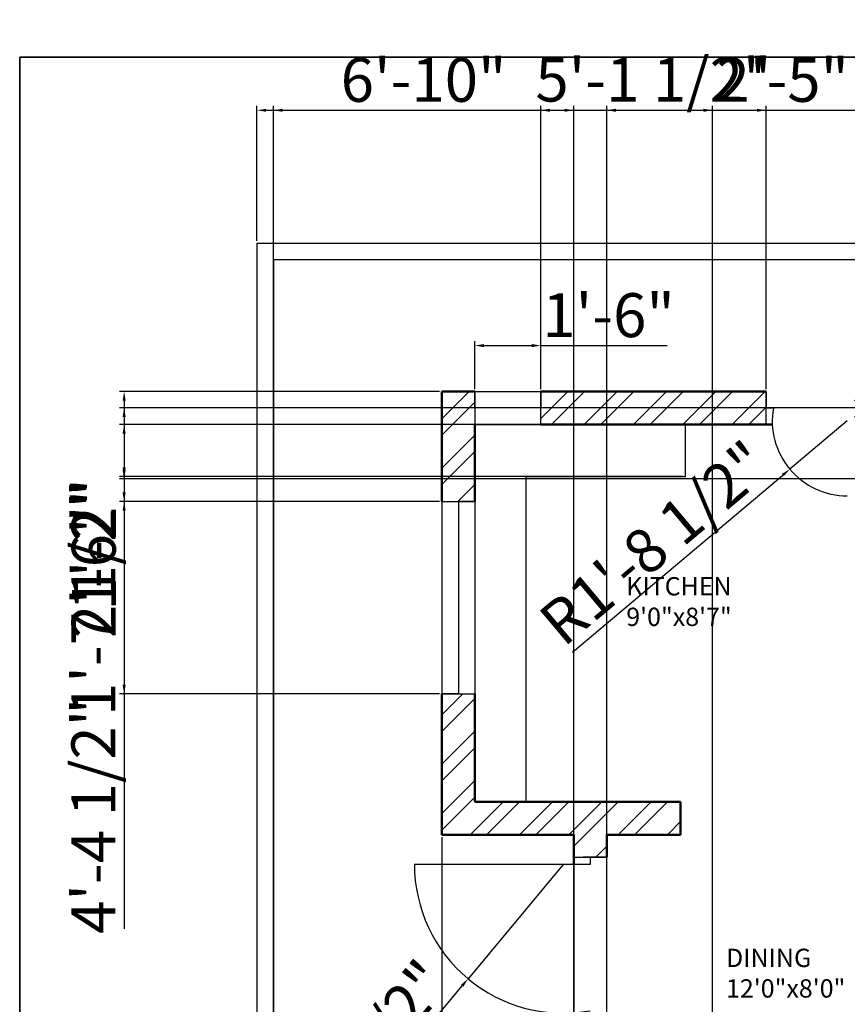
# Model space of a CAD drawing. Units: inches. Extents: x 1990 to 2869, y 1755 to 2533.
# Tile 2 of 6: x 1990 to 2216, y 2120 to 2389. Entities that reach past the tile are written whole.
import ezdxf

# ---------------------------------------------------------------- set-up
doc = ezdxf.new("R2010")
doc.units = ezdxf.units.IN
for name, color, linetype, lineweight in [('A-ANNO-DIMS', 171, 'Continuous', 18), ('A-ANNO-TTLB', 7, 'Continuous', 35), ('A-AREA-IDEN', 7, 'Continuous', 18), ('A-DOOR', 11, 'Continuous', 25), ('A-FLOR-CASE', 7, 'Continuous', 25), ('A-GLAZ', 121, 'Continuous', 25), ('A-WALL', 7, 'Continuous', 50), ('A-WALL-SITE', 7, 'Continuous', 30)]:
    doc.layers.add(name, color=color, linetype=linetype, lineweight=lineweight)
doc.layers.add('A-WALL-PATT', color=215, linetype='Continuous', lineweight=13, true_color=0xa953a0)
doc.styles.get("Standard").update_dxf_attribs({"font": 'arial.ttf'})
doc.dimstyles.new('ISO-25', dxfattribs={"dimtxt": 12, "dimasz": 2.5, "dimexe": 1.25, "dimexo": 0.625, "dimtad": 1, "dimdec": 0, "dimlunit": 3, "dimtxsty": 'Standard', "dimcen": 2.5, "dimadec": 0, "dimazin": 0, "dimtfac": 1, "dimtdec": 0, "dimtmove": 0, "dimatfit": 3, "dimfxl": 1, "dimarcsym": 0})

# ---------------------------------------------------------------- blocks, each defined once
blk = doc.blocks.new('*D2')
at = {"layer": 'A-ANNO-DIMS', "color": 0, "lineweight": -2, "transparency": 16777216}
for p, q in [((2113.97, 2288.18), (2113.97, 2301.32)), ((2131.97, 2288.18), (2131.97, 2301.32)), ((2116.47, 2300.07), (2129.47, 2300.07)), ((2131.97, 2300.07), (2166.49, 2300.07))]:
    blk.add_line(p, q, dxfattribs=at)
at = {"layer": 'A-ANNO-DIMS', "color": 0, "transparency": 16777216}
for points in [[(2116.47, 2300.49), (2116.47, 2299.65), (2113.97, 2300.07)], [(2129.47, 2300.49), (2129.47, 2299.65), (2131.97, 2300.07)]]:
    blk.add_solid(points, dxfattribs=at)
at = {"layer": 'Defpoints', "color": 0, "transparency": 16777216}
for p in [(2131.97, 2300.07), (2113.97, 2287.55), (2131.97, 2287.55)]:
    blk.add_point(p, dxfattribs=at)
at = {"layer": 'A-ANNO-DIMS', "color": 0, "transparency": 16777216, "insert": (2150.48, 2306.82), "char_height": 12, "attachment_point": 5}
blk.add_mtext('1\'-6"', dxfattribs=at)
blk = doc.blocks.new('WIN-18IN')
for p, q in [((0, 4.5), (0, 9)), ((0, 9), (0, 0)), ((0, 9), (18, 9)), ((18, 0), (18, 9)), ((18, 9), (18, 4.5)), ((18, 4.5), (0, 4.5)), ((0, 0), (18, 0))]:
    blk.add_line(p, q)
blk = doc.blocks.new('*D24')
at = {"layer": 'A-ANNO-DIMS', "color": 0, "lineweight": -2, "transparency": 16777216}
for p, q in [((2149.97, 1894.18), (2149.97, 2365.55)), ((2178.84, 1894.18), (2178.84, 2365.55)), ((2152.47, 2364.3), (2176.34, 2364.3)), ((2178.84, 2364.3), (2214.69, 2364.3))]:
    blk.add_line(p, q, dxfattribs=at)
at = {"layer": 'A-ANNO-DIMS', "color": 0, "transparency": 16777216}
for points in [[(2152.47, 2364.72), (2152.47, 2363.88), (2149.97, 2364.3)], [(2176.34, 2364.72), (2176.34, 2363.88), (2178.84, 2364.3)]]:
    blk.add_solid(points, dxfattribs=at)
at = {"layer": 'Defpoints', "color": 0, "transparency": 16777216}
for p in [(2178.84, 2364.3), (2149.97, 1893.55), (2178.84, 1893.55)]:
    blk.add_point(p, dxfattribs=at)
at = {"layer": 'A-ANNO-DIMS', "color": 0, "transparency": 16777216, "insert": (2198.02, 2371.05), "char_height": 12, "attachment_point": 5}
blk.add_mtext('2\'-5"', dxfattribs=at)
blk = doc.blocks.new('*D25')
at = {"layer": 'A-ANNO-DIMS', "color": 0, "lineweight": -2, "transparency": 16777216}
for p, q in [((2058.97, 1885.18), (2058.97, 2365.55)), ((2140.97, 1885.18), (2140.97, 2365.55)), ((2061.47, 2364.3), (2138.47, 2364.3))]:
    blk.add_line(p, q, dxfattribs=at)
at = {"layer": 'A-ANNO-DIMS', "color": 0, "transparency": 16777216}
for points in [[(2061.47, 2364.72), (2061.47, 2363.88), (2058.97, 2364.3)], [(2138.47, 2364.72), (2138.47, 2363.88), (2140.97, 2364.3)]]:
    blk.add_solid(points, dxfattribs=at)
at = {"layer": 'Defpoints', "color": 0, "transparency": 16777216}
for p in [(2140.97, 2364.3), (2058.97, 1884.55), (2140.97, 1884.55)]:
    blk.add_point(p, dxfattribs=at)
at = {"layer": 'A-ANNO-DIMS', "color": 0, "transparency": 16777216, "insert": (2099.97, 2371.05), "char_height": 12, "attachment_point": 5}
blk.add_mtext('6\'-10"', dxfattribs=at)
blk = doc.blocks.new('*D33')
at = {"layer": 'A-ANNO-DIMS', "color": 0, "lineweight": -2, "transparency": 16777216}
for p, q in [((2104.97, 2165.93), (2104.97, 1764.83)), ((2140.97, 2165.93), (2140.97, 1764.83)), ((2107.47, 1766.08), (2138.47, 1766.08))]:
    blk.add_line(p, q, dxfattribs=at)
at = {"layer": 'A-ANNO-DIMS', "color": 0, "transparency": 16777216}
for points in [[(2107.47, 1766.49), (2107.47, 1765.66), (2104.97, 1766.08)], [(2138.47, 1766.49), (2138.47, 1765.66), (2140.97, 1766.08)]]:
    blk.add_solid(points, dxfattribs=at)
at = {"layer": 'Defpoints', "color": 0, "transparency": 16777216}
for p in [(2104.97, 2166.55), (2140.97, 2166.55), (2140.97, 1766.08)]:
    blk.add_point(p, dxfattribs=at)
at = {"layer": 'A-ANNO-DIMS', "color": 0, "transparency": 16777216, "insert": (2122.97, 1772.83), "char_height": 12, "attachment_point": 5}
blk.add_mtext('3\'-0"', dxfattribs=at)
blk = doc.blocks.new('*D34')
at = {"layer": 'A-ANNO-DIMS', "color": 0, "lineweight": -2, "transparency": 16777216}
for p, q in [((2104.35, 2257.5), (2016.97, 2257.5)), ((2018.22, 2255), (2018.22, 2207.5)), ((2104.35, 2205), (2016.97, 2205)), ((2018.22, 2205), (2018.22, 2140.9))]:
    blk.add_line(p, q, dxfattribs=at)
at = {"layer": 'A-ANNO-DIMS', "color": 0, "transparency": 16777216}
for points in [[(2017.8, 2255), (2018.64, 2255), (2018.22, 2257.5)], [(2017.8, 2207.5), (2018.64, 2207.5), (2018.22, 2205)]]:
    blk.add_solid(points, dxfattribs=at)
at = {"layer": 'Defpoints', "color": 0, "transparency": 16777216}
for p in [(2104.97, 2257.5), (2018.22, 2205), (2104.97, 2205)]:
    blk.add_point(p, dxfattribs=at)
at = {"layer": 'A-ANNO-DIMS', "color": 0, "transparency": 16777216, "insert": (2011.39, 2171.7), "char_height": 12, "attachment_point": 5, "rotation": 90}
blk.add_mtext('4\'-4 1/2"', dxfattribs=at)
blk = doc.blocks.new('*D35')
at = {"layer": 'A-ANNO-DIMS', "color": 0, "lineweight": -2, "transparency": 16777216}
for p, q in [((2104.35, 2287.55), (2016.97, 2287.55)), ((2018.22, 2285.05), (2018.22, 2260)), ((2104.35, 2257.5), (2016.97, 2257.5)), ((2018.22, 2257.5), (2018.22, 2221.64))]:
    blk.add_line(p, q, dxfattribs=at)
at = {"layer": 'A-ANNO-DIMS', "color": 0, "transparency": 16777216}
for points in [[(2017.8, 2285.05), (2018.64, 2285.05), (2018.22, 2287.55)], [(2017.8, 2260), (2018.64, 2260), (2018.22, 2257.5)]]:
    blk.add_solid(points, dxfattribs=at)
at = {"layer": 'Defpoints', "color": 0, "transparency": 16777216}
for p in [(2104.97, 2287.55), (2018.22, 2257.5), (2104.97, 2257.5)]:
    blk.add_point(p, dxfattribs=at)
at = {"layer": 'A-ANNO-DIMS', "color": 0, "transparency": 16777216, "insert": (2011.47, 2238.32), "char_height": 12, "attachment_point": 5, "rotation": 90}
blk.add_mtext('2\'-6"', dxfattribs=at)
blk = doc.blocks.new('*D36')
at = {"layer": 'A-ANNO-DIMS', "color": 0, "lineweight": -2, "transparency": 16777216}
for p, q in [((2716.35, 2283.05), (2016.97, 2283.05)), ((2018.22, 2280.55), (2018.22, 2266.18)), ((2716.35, 2263.68), (2016.97, 2263.68)), ((2018.22, 2263.68), (2018.22, 2201.19))]:
    blk.add_line(p, q, dxfattribs=at)
at = {"layer": 'A-ANNO-DIMS', "color": 0, "transparency": 16777216}
for points in [[(2017.8, 2280.55), (2018.64, 2280.55), (2018.22, 2283.05)], [(2017.8, 2266.18), (2018.64, 2266.18), (2018.22, 2263.68)]]:
    blk.add_solid(points, dxfattribs=at)
at = {"layer": 'Defpoints', "color": 0, "transparency": 16777216}
for p in [(2716.97, 2283.05), (2018.22, 2263.68), (2716.97, 2263.68)]:
    blk.add_point(p, dxfattribs=at)
at = {"layer": 'A-ANNO-DIMS', "color": 0, "transparency": 16777216, "insert": (2011.39, 2231.19), "char_height": 12, "attachment_point": 5, "rotation": 90}
blk.add_mtext('1\'-7 1/2"', dxfattribs=at)
blk = doc.blocks.new('*D42')
at = {"layer": 'A-ANNO-DIMS', "color": 0, "lineweight": -2, "transparency": 16777216}
for p, q in [((2170.81, 2278.55), (2016.97, 2278.55)), ((2018.22, 2276.05), (2018.22, 2266.83)), ((2170.81, 2264.33), (2016.97, 2264.33)), ((2018.22, 2264.33), (2018.22, 2229.81))]:
    blk.add_line(p, q, dxfattribs=at)
at = {"layer": 'A-ANNO-DIMS', "color": 0, "transparency": 16777216}
for points in [[(2017.8, 2276.05), (2018.64, 2276.05), (2018.22, 2278.55)], [(2017.8, 2266.83), (2018.64, 2266.83), (2018.22, 2264.33)]]:
    blk.add_solid(points, dxfattribs=at)
at = {"layer": 'Defpoints', "color": 0, "transparency": 16777216}
for p in [(2171.44, 2278.55), (2018.22, 2264.33), (2171.44, 2264.33)]:
    blk.add_point(p, dxfattribs=at)
at = {"layer": 'A-ANNO-DIMS', "color": 0, "transparency": 16777216, "insert": (2011.57, 2245.82), "char_height": 12, "attachment_point": 5, "rotation": 90}
blk.add_mtext('1\'-2"', dxfattribs=at)
blk = doc.blocks.new('*D45')
at = {"layer": 'A-ANNO-DIMS', "color": 0, "lineweight": -2, "transparency": 16777216}
for p, q in [((2131.97, 2288.18), (2131.97, 2365.55)), ((2193.46, 2288.18), (2193.46, 2365.55)), ((2134.47, 2364.3), (2190.96, 2364.3))]:
    blk.add_line(p, q, dxfattribs=at)
at = {"layer": 'A-ANNO-DIMS', "color": 0, "transparency": 16777216}
for points in [[(2134.47, 2364.72), (2134.47, 2363.88), (2131.97, 2364.3)], [(2190.96, 2364.72), (2190.96, 2363.88), (2193.46, 2364.3)]]:
    blk.add_solid(points, dxfattribs=at)
at = {"layer": 'Defpoints', "color": 0, "transparency": 16777216}
for p in [(2193.46, 2364.3), (2131.97, 2287.55), (2193.46, 2287.55)]:
    blk.add_point(p, dxfattribs=at)
at = {"layer": 'A-ANNO-DIMS', "color": 0, "transparency": 16777216, "insert": (2162.72, 2371.13), "char_height": 12, "attachment_point": 5}
blk.add_mtext('5\'-1 1/2"', dxfattribs=at)
blk = doc.blocks.new('*D48')
at = {"layer": 'A-ANNO-DIMS', "color": 0, "lineweight": -2, "transparency": 16777216}
for p, q in [((2054.47, 2328.68), (2054.47, 2365.55)), ((2776.47, 2328.68), (2776.47, 2365.55)), ((2056.97, 2364.3), (2773.97, 2364.3))]:
    blk.add_line(p, q, dxfattribs=at)
at = {"layer": 'A-ANNO-DIMS', "color": 0, "transparency": 16777216}
for points in [[(2056.97, 2364.72), (2056.97, 2363.88), (2054.47, 2364.3)], [(2773.97, 2364.72), (2773.97, 2363.88), (2776.47, 2364.3)]]:
    blk.add_solid(points, dxfattribs=at)
at = {"layer": 'Defpoints', "color": 0, "transparency": 16777216}
for p in [(2776.47, 2364.3), (2054.47, 2328.05), (2776.47, 2328.05)]:
    blk.add_point(p, dxfattribs=at)
at = {"layer": 'A-ANNO-DIMS', "color": 0, "transparency": 16777216, "insert": (2415.47, 2371.05), "char_height": 12, "attachment_point": 5}
blk.add_mtext('60\'-2"', dxfattribs=at)
blk = doc.blocks.new('*D50')
at = {"layer": 'A-ANNO-DIMS', "color": 0, "lineweight": -2, "transparency": 16777216}
for p, q in [((2138.1, 2158.48), (2112.11, 2127.26)), ((2062.46, 2067.62), (2110.51, 2125.33))]:
    blk.add_line(p, q, dxfattribs=at)
at = {"layer": 'A-ANNO-DIMS', "color": 0, "transparency": 16777216}
blk.add_solid([(2110.19, 2125.6), (2110.83, 2125.07), (2112.11, 2127.26)], dxfattribs=at)
at = {"layer": 'Defpoints', "color": 0, "transparency": 16777216}
for p in [(2138.1, 2158.48), (2112.11, 2127.26)]:
    blk.add_point(p, dxfattribs=at)
at = {"layer": 'A-ANNO-DIMS', "color": 0, "transparency": 16777216, "insert": (2080.43, 2099.89), "char_height": 12, "attachment_point": 5, "rotation": 50.2228}
blk.add_mtext('R3\'-4 1/2"', dxfattribs=at)
blk = doc.blocks.new('*D58')
at = {"layer": 'A-ANNO-DIMS', "color": 0, "lineweight": -2, "transparency": 16777216}
for p, q in [((2215.66, 2279.55), (2199.98, 2266.35)), ((2140.6, 2216.39), (2198.06, 2264.74))]:
    blk.add_line(p, q, dxfattribs=at)
at = {"layer": 'A-ANNO-DIMS', "color": 0, "transparency": 16777216}
blk.add_solid([(2197.79, 2265.06), (2198.33, 2264.42), (2199.98, 2266.35)], dxfattribs=at)
at = {"layer": 'Defpoints', "color": 0, "transparency": 16777216}
for p in [(2215.66, 2279.55), (2199.98, 2266.35)]:
    blk.add_point(p, dxfattribs=at)
at = {"layer": 'A-ANNO-DIMS', "color": 0, "transparency": 16777216, "insert": (2163.98, 2244.99), "char_height": 12, "attachment_point": 5, "rotation": 40.0794}
blk.add_mtext('R1\'-8 1/2"', dxfattribs=at)

msp = doc.modelspace()

# ---------------------------------------------------------------- hatches: boundary and pattern name
at = {"layer": 'A-WALL-PATT'}
h = msp.add_hatch(dxfattribs=at)
h.set_pattern_fill('ANSI32', color=256)
h.paths.add_polyline_path([(2193.46, 2287.55), (2131.97, 2287.55), (2131.97, 2278.55), (2193.46, 2278.55)])
h.paths.add_polyline_path([(2113.97, 2278.55), (2113.97, 2287.55), (2104.97, 2287.55), (2104.97, 2257.5), (2113.97, 2257.5)])
h.paths.add_polyline_path([(2113.97, 2205), (2104.97, 2205), (2104.97, 2166.55), (2140.97, 2166.55), (2140.97, 2160.48), (2149.97, 2160.48), (2149.97, 2166.55), (2170.14, 2166.55), (2170.14, 2175.55), (2113.97, 2175.55)])
h.paths.add_polyline_path([(2278.97, 2287.55), (2244.47, 2287.55), (2244.47, 2278.55), (2274.47, 2278.55), (2274.47, 2200.55), (2226.47, 2200.55), (2226.47, 2219.37), (2221.97, 2219.37), (2221.97, 2175.55), (2221.97, 2166.55), (2226.47, 2166.55), (2226.47, 2196.05), (2274.47, 2196.05), (2274.47, 2166.55), (2284.01, 2166.55), (2284.01, 2171.05), (2284.01, 2175.55), (2278.97, 2175.55), (2278.97, 2278.55)])
h.paths.add_polyline_path([(2226.47, 2283.05), (2226.47, 2287.55), (2217.66, 2287.55), (2217.66, 2283.05), (2217.66, 2278.55), (2221.97, 2278.55), (2221.97, 2255.21), (2226.47, 2255.21), (2226.47, 2278.55)])
h.paths.add_polyline_path([(2560.97, 2328.05), (2551.97, 2328.05), (2269.97, 2328.05), (2269.97, 2319.05), (2278.97, 2319.05), (2410.97, 2319.05), (2410.97, 2187.05), (2346.47, 2187.05), (2346.47, 2175.55), (2319.77, 2175.55), (2319.77, 2166.55), (2346.47, 2166.55), (2346.47, 2128.22), (2350.97, 2128.22), (2350.97, 2178.05), (2410.97, 2178.05), (2410.97, 2175.55), (2410.97, 2106.05), (2350.97, 2106.05), (2350.97, 2108.72), (2348.72, 2108.72), (2346.47, 2108.72), (2346.47, 2106.05), (2342.3, 2106.05), (2342.3, 2097.05), (2346.47, 2097.05), (2350.97, 2097.05), (2410.97, 2097.05), (2410.97, 1974.05), (2373.73, 1974.05), (2373.73, 1965.05), (2419.97, 1965.05), (2447.99, 1965.05), (2447.99, 1969.55), (2447.99, 1974.05), (2419.97, 1974.05), (2419.97, 2097.05), (2484.47, 2097.05), (2489.55, 2097.05), (2489.55, 2106.05), (2484.47, 2106.05), (2484.47, 2108.84), (2482.22, 2108.84), (2479.97, 2108.84), (2479.97, 2106.05), (2419.97, 2106.05), (2419.97, 2175.55), (2419.97, 2178.05), (2479.97, 2178.05), (2479.97, 2128.49), (2484.47, 2128.49), (2484.47, 2166.55), (2511.88, 2166.55), (2511.88, 2171.05), (2511.88, 2175.55), (2484.47, 2175.55), (2484.47, 2187.05), (2479.97, 2187.05), (2419.97, 2187.05), (2419.97, 2319.05), (2551.97, 2319.05), (2560.97, 2319.05)])
h.paths.add_polyline_path([(2586.47, 2292.05), (2560.97, 2292.05), (2551.97, 2292.05), (2551.97, 2175.55), (2547.37, 2175.55), (2547.37, 2166.55), (2556.47, 2166.55), (2556.47, 2175.55), (2556.47, 2205.05), (2604.47, 2205.05), (2604.47, 2166.55), (2608.97, 2166.55), (2608.97, 2175.55), (2608.97, 2205.05), (2608.97, 2228.1), (2604.47, 2228.1), (2604.47, 2209.55), (2556.47, 2209.55), (2556.47, 2283.05), (2586.47, 2283.05)])
h.paths.add_polyline_path([(2691.55, 2292.05), (2690.86, 2292.05), (2636.82, 2292.05), (2636.82, 2283.05), (2691.55, 2283.05)])
h.paths.add_polyline_path([(2725.97, 2292.05), (2716.97, 2292.05), (2709.55, 2292.05), (2709.55, 2287.55), (2709.55, 2283.05), (2716.97, 2283.05), (2716.97, 2263.68), (2725.97, 2263.68)])
h.paths.add_polyline_path([(2725.97, 2199.18), (2716.97, 2199.18), (2716.97, 2180.05), (2716.97, 2175.55), (2650.43, 2175.55), (2650.43, 2166.55), (2680.97, 2166.55), (2680.97, 2159.77), (2689.97, 2159.77), (2689.97, 2166.55), (2725.97, 2166.55)])
h.paths.add_polyline_path([(2536.97, 2061.55), (2554.82, 2061.55), (2554.82, 2070.55), (2536.97, 2070.55), (2536.97, 2097.05), (2536.97, 2106.05), (2524.42, 2106.05), (2524.42, 2101.55), (2524.42, 2097.05), (2527.97, 2097.05), (2527.97, 1974.05), (2497.49, 1974.05), (2497.49, 1965.05), (2527.97, 1965.05), (2527.97, 1929.96), (2536.97, 1929.96)])
h.paths.add_polyline_path([(2689.97, 1945.55), (2685.47, 1945.55), (2680.97, 1945.55), (2680.97, 1893.55), (2625.68, 1893.55), (2625.68, 1884.55), (2689.97, 1884.55), (2689.97, 1893.55)])
h.paths.add_polyline_path([(2168.89, 2070.55), (2149.97, 2070.55), (2149.97, 2116.52), (2145.47, 2116.52), (2140.97, 2116.52), (2140.97, 1977.7), (2145.47, 1977.7), (2145.47, 1977.63), (2149.97, 1977.55), (2149.97, 2061.55), (2168.89, 2061.55)])
h.paths.add_polyline_path([(2302.97, 2097.05), (2306.2, 2097.05), (2306.2, 2106.05), (2293.97, 2106.05), (2293.97, 2097.05), (2293.97, 2070.55), (2269.93, 2070.55), (2269.93, 2061.55), (2293.97, 2061.55), (2293.97, 1930.78), (2302.97, 1930.78), (2302.97, 1965.05), (2324.23, 1965.05), (2324.23, 1969.55), (2324.23, 1974.05), (2302.97, 1974.05)])
h.paths.add_polyline_path([(2149.97, 1928.2), (2145.47, 1928.2), (2140.97, 1928.2), (2140.97, 1889.05), (2140.97, 1884.55), (2178.84, 1884.55), (2178.84, 1889.05), (2178.84, 1893.55), (2149.97, 1893.55)])
h.paths.add_polyline_path([(2302.97, 1898.24), (2298.47, 1898.24), (2293.97, 1898.24), (2293.97, 1893.55), (2243.34, 1893.55), (2243.34, 1884.55), (2302.97, 1884.55)])

# ---------------------------------------------------------------- linework, layer by layer
at = {"layer": 'A-ANNO-TTLB'}
msp.add_lwpolyline([(1989.71, 2378.83), (2869.46, 2378.83), (2869.46, 1755.45), (1989.71, 1755.45)], close=True, dxfattribs=at)
at = {"layer": 'A-DOOR'}
for p, q in [((2193.46, 2278.55), (2193.46, 2287.55)), ((2193.46, 2287.55), (2193.46, 2283.05)), ((2193.46, 2283.05), (2195.46, 2283.05)), ((2145.47, 2158.48), (2097.47, 2158.48)), ((2140.97, 2160.48), (2149.97, 2160.48)), ((2149.97, 2160.48), (2143.5, 2160.48)), ((2145.47, 2160.48), (2145.47, 2158.48))]:
    msp.add_line(p, q, dxfattribs=at)
for centre, radius, start, end in [((2215.66, 2279.55), 20.5, 170.1581, 270), ((2138.1, 2158.48), 40.63, 180, 280.4464)]:
    msp.add_arc(centre, radius, start, end, dxfattribs=at)
at = {"layer": 'A-FLOR-CASE'}
for p, q in [((2171.44, 2264.33), (2171.44, 2278.55)), ((2127.94, 2175.55), (2127.94, 2264.33)), ((2127.94, 2264.33), (2171.44, 2264.33))]:
    msp.add_line(p, q, dxfattribs=at)
at = {"layer": 'A-GLAZ'}
for p, q in [((2104.97, 2257.5), (2113.97, 2257.5)), ((2104.97, 2257.5), (2104.97, 2205)), ((2113.97, 2257.5), (2109.47, 2257.5)), ((2109.47, 2257.5), (2109.47, 2205)), ((2113.97, 2257.5), (2113.97, 2205)), ((2109.47, 2205), (2104.97, 2205)), ((2104.97, 2205), (2113.97, 2205))]:
    msp.add_line(p, q, dxfattribs=at)
at = {"layer": 'A-WALL'}
for p, q in [((2104.97, 2287.55), (2113.97, 2287.55)), ((2104.97, 2287.55), (2104.97, 2257.5)), ((2131.97, 2287.55), (2193.46, 2287.55)), ((2113.97, 2278.55), (2113.97, 2257.5)), ((2131.97, 2278.55), (2195.19, 2278.55)), ((2104.97, 2205), (2104.97, 2166.55)), ((2113.97, 2205), (2113.97, 2175.55)), ((2113.97, 2175.55), (2170.14, 2175.55)), ((2170.14, 2175.55), (2170.14, 2166.55)), ((2104.97, 2166.55), (2140.97, 2166.55)), ((2140.97, 2166.55), (2140.97, 2158.48)), ((2149.97, 2166.55), (2149.97, 2160.48)), ((2149.97, 2166.55), (2170.14, 2166.55))]:
    msp.add_line(p, q, dxfattribs=at)
at = {"layer": 'A-WALL-SITE'}
for p, q in [((2054.47, 2328.05), (2776.47, 2328.05)), ((2054.47, 2328.05), (2054.47, 1884.55)), ((2058.97, 2323.55), (2269.97, 2323.55)), ((2058.97, 2323.55), (2058.97, 1889.05))]:
    msp.add_line(p, q, dxfattribs=at)

# ---------------------------------------------------------------- block references
at = {"layer": 'A-GLAZ'}
msp.add_blockref('WIN-18IN', (2113.97, 2278.55), dxfattribs=at)

# ---------------------------------------------------------------- texts
at = {"layer": 'A-AREA-IDEN', "char_height": 5, "attachment_point": 1}
for s, width, insert in [('KITCHEN \\P9\'0"x8\'7"', 151.5227, (2155.31, 2236.87)), ('DINING\\P12\'0"x8\'0"', 140.2747, (2182.55, 2135.45))]:
    msp.add_mtext_dynamic_manual_height_columns(s, width=width, gutter_width=12.5, heights=[0], dxfattribs=dict(at, insert=insert))

# ---------------------------------------------------------------- dimensions: what is measured, and where the dimension line sits
at = {"layer": 'A-ANNO-DIMS'}
for base, p1, p2, override, picture, middle in [((2193.46, 2364.3), (2131.97, 2287.55), (2193.46, 2287.55), {"dimdec": 1, "dimlfac": 1, "dimrnd": 0, "dimzin": 1, "dimdsep": 46, "dimlunit": 4, "dimfrac": 2}, '*D45', (2162.72, 2371.13)), ((2776.47, 2364.3), (2054.47, 2328.05), (2776.47, 2328.05), {"dimdec": 1, "dimlfac": 1, "dimrnd": 0, "dimzin": 1, "dimdsep": 46, "dimlunit": 4, "dimfrac": 2}, '*D48', (2415.47, 2371.05)), ((2140.97, 2364.3), (2058.97, 1884.55), (2140.97, 1884.55), {"dimdec": 1, "dimlfac": 1, "dimrnd": 0, "dimzin": 1, "dimdsep": 46, "dimlunit": 4, "dimfrac": 2}, '*D25', (2099.97, 2371.05)), ((2178.84, 2364.3), (2149.97, 1893.55), (2178.84, 1893.55), {"dimdec": 1, "dimlfac": 1, "dimrnd": 0, "dimzin": 1, "dimdsep": 46, "dimlunit": 4, "dimfrac": 2}, '*D24', (2198.02, 2371.05)), ((2131.97, 2300.07), (2113.97, 2287.55), (2131.97, 2287.55), {"dimclrd": 0, "dimclre": 0, "dimclrt": 0}, '*D2', (2150.48, 2306.82)), ((2140.97, 1766.08), (2104.97, 2166.55), (2140.97, 2166.55), {"dimdec": 1, "dimlfac": 1, "dimrnd": 0, "dimzin": 1, "dimdsep": 46, "dimlunit": 4, "dimfrac": 2}, '*D33', (2122.97, 1772.83))]:
    dim = msp.add_linear_dim(base=base, p1=p1, p2=p2, dimstyle='ISO-25', override=override, dxfattribs=at)
    dim.commit()
    dim.dimension.update_dxf_attribs({"geometry": picture, "text_midpoint": middle})
for base, p1, p2, picture, middle in [((2018.2213, 2257.4965), (2104.9713, 2287.5512), (2104.9713, 2257.4965), '*D35', (2011.4695, 2238.3196)), ((2018.22, 2263.68), (2716.97, 2283.05), (2716.97, 2263.68), '*D36', (2011.39, 2231.19)), ((2018.22, 2264.33), (2171.44, 2278.55), (2171.44, 2264.33), '*D42', (2011.57, 2245.82)), ((2018.22, 2205), (2104.97, 2257.5), (2104.97, 2205), '*D34', (2011.39, 2171.7))]:
    dim = msp.add_linear_dim(base=base, p1=p1, p2=p2, angle=90, dimstyle='ISO-25', override={"dimdec": 1, "dimlfac": 1, "dimrnd": 0, "dimzin": 1, "dimdsep": 46, "dimlunit": 4, "dimfrac": 2}, dxfattribs=at)
    dim.commit()
    dim.dimension.update_dxf_attribs({"geometry": picture, "text_midpoint": middle})
for center, mpoint, picture, middle in [((2215.66, 2279.55), (2199.98, 2266.35), '*D58', (2163.98, 2244.99)), ((2138.1, 2158.48), (2112.11, 2127.26), '*D50', (2080.43, 2099.89))]:
    dim = msp.add_radius_dim(center=center, mpoint=mpoint, dimstyle='ISO-25', override={"dimdec": 1, "dimlfac": 1, "dimrnd": 0, "dimzin": 1, "dimdsep": 46, "dimlunit": 4, "dimfrac": 2}, dxfattribs=at)
    dim.commit()
    dim.dimension.update_dxf_attribs({"geometry": picture, "text_midpoint": middle})

doc.saveas('drawing.dxf')
